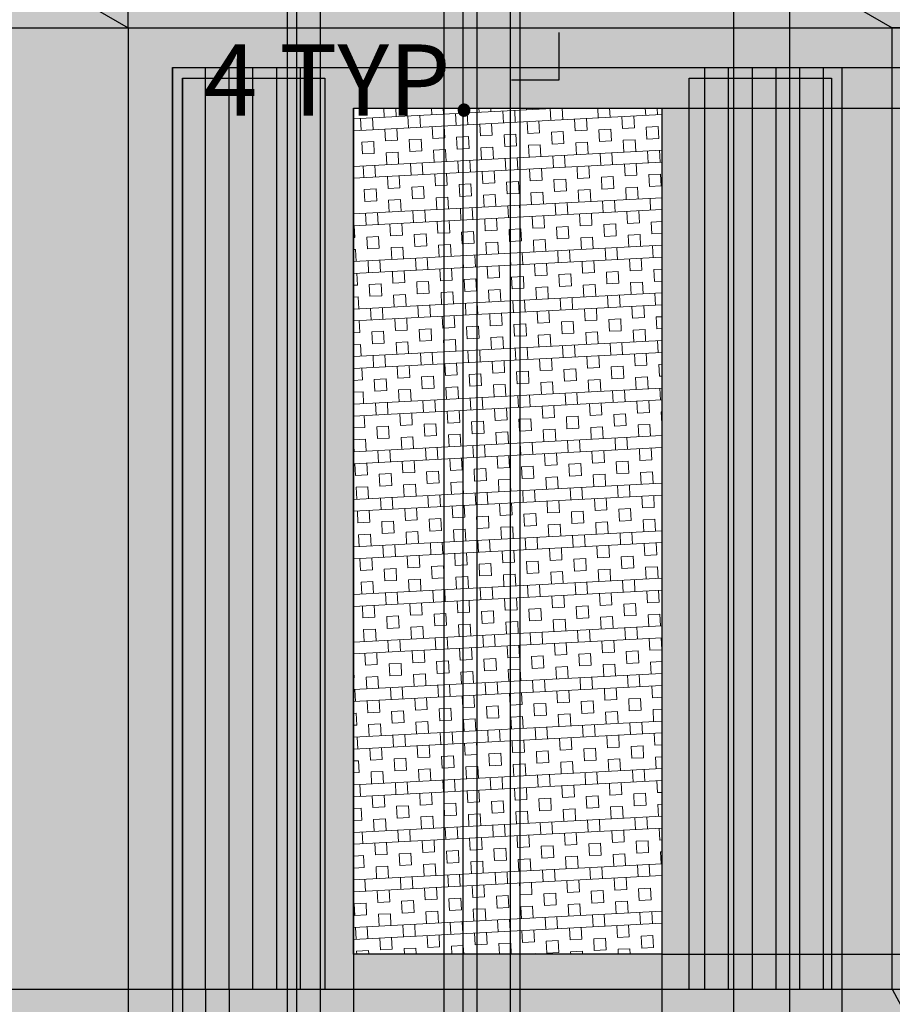
# Model space of a CAD drawing. Units: millimetres. Extents: x 131 to 845, y -20 to 1043.
# Tile 4 of 11: x 467 to 651, y 95 to 302. Entities that reach past the tile are written whole.
import ezdxf

# ---------------------------------------------------------------- set-up
doc = ezdxf.new("R2010")
doc.units = ezdxf.units.MM
doc.header["$MEASUREMENT"] = 0
for name, color, linetype, lineweight in [('A-ANNO-DIMS', 2, 'Continuous', 18), ('A-DOOR', 3, 'Continuous', 25), ('A-ELEV', 7, 'Continuous', 25), ('A-ELEV-PATT', 7, 'Continuous', 13), ('A-ELEV-SCRN', 4, 'Continuous', 13), ('A-GLAZ-PATT', 143, 'Continuous', 13)]:
    doc.layers.add(name, color=color, linetype=linetype, lineweight=lineweight)
doc.styles.get("Standard").update_dxf_attribs({"font": 'arial.ttf'})
doc.dimstyles.get("Standard").update_dxf_attribs({"dimtxt": 15, "dimasz": 10, "dimexe": 0.18, "dimexo": 0.0625, "dimgap": 5, "dimtad": 0, "dimtih": 1, "dimtoh": 1, "dimdec": 0, "dimzin": 0, "dimdsep": 46, "dimtxsty": 'Standard', "dimcen": 5, "dimadec": 0, "dimazin": 0, "dimtfac": 1, "dimtdec": 0, "dimtofl": 0, "dimtmove": 0, "dimatfit": 3, "dimfxl": 1, "dimtolj": 1, "dimtzin": 0, "dimarcsym": 0})

# ---------------------------------------------------------------- blocks, each defined once
blk = doc.blocks.new('*D9')
at = {"layer": 'A-ANNO-DIMS', "color": 0, "lineweight": -2, "transparency": 16777216}
for p, q in [((571.05, 313.91), (561.05, 313.91)), ((581.05, 313.22), (581.05, 314.09)), ((586.05, 313.22), (586.05, 314.09)), ((596.05, 313.91), (606.05, 313.91))]:
    blk.add_line(p, q, dxfattribs=at)
at = {"layer": 'A-ANNO-DIMS', "color": 0, "transparency": 16777216}
for points in [[(571.05, 315.58), (571.05, 312.24), (581.05, 313.91)], [(596.05, 315.58), (596.05, 312.24), (586.05, 313.91)]]:
    blk.add_solid(points, dxfattribs=at)
at = {"layer": 'Defpoints', "color": 0, "transparency": 16777216}
for p in [(581.05, 313.91), (581.05, 313.16), (586.05, 313.16)]:
    blk.add_point(p, dxfattribs=at)
at = {"layer": 'A-ANNO-DIMS', "color": 0, "transparency": 16777216, "insert": (409.24, 313.91), "char_height": 15, "attachment_point": 5}
blk.add_mtext('\\A1;BALCONY RAIL PANEL 5 TYP.', dxfattribs=at)
blk = doc.blocks.new('*D10')
at = {"layer": 'A-ANNO-DIMS', "color": 0, "lineweight": -2, "transparency": 16777216}
for p, q in [((580.3, 323.16), (580.3, 333.16)), ((580.98, 313.16), (580.12, 313.16)), ((580.98, 309.16), (580.12, 309.16)), ((580.3, 299.16), (580.3, 289.16)), ((580.3, 289.16), (570.3, 289.16))]:
    blk.add_line(p, q, dxfattribs=at)
at = {"layer": 'A-ANNO-DIMS', "color": 0, "transparency": 16777216}
for points in [[(578.63, 323.16), (581.96, 323.16), (580.3, 313.16)], [(578.63, 299.16), (581.96, 299.16), (580.3, 309.16)]]:
    blk.add_solid(points, dxfattribs=at)
at = {"layer": 'Defpoints', "color": 0, "transparency": 16777216}
for p in [(581.05, 313.16), (580.3, 309.16), (581.05, 309.16)]:
    blk.add_point(p, dxfattribs=at)
at = {"layer": 'A-ANNO-DIMS', "color": 0, "transparency": 16777216, "insert": (534.31, 289.16), "char_height": 15, "attachment_point": 5}
blk.add_mtext('\\A1;4 TYP.', dxfattribs=at)
blk = doc.blocks.new('*D50')
at = {"layer": 'A-ANNO-DIMS', "color": 0, "lineweight": -2, "transparency": 16777216}
for p, q in [((720.6, 488.6), (768.56, 488.6)), ((768.38, 478.6), (768.38, 287.12)), ((768.38, 70.31), (768.38, 261.79)), ((216.3, 60.31), (768.56, 60.31))]:
    blk.add_line(p, q, dxfattribs=at)
at = {"layer": 'A-ANNO-DIMS', "color": 0, "transparency": 16777216}
for points in [[(766.72, 478.6), (770.05, 478.6), (768.38, 488.6)], [(766.72, 70.31), (770.05, 70.31), (768.38, 60.31)]]:
    blk.add_solid(points, dxfattribs=at)
at = {"layer": 'Defpoints', "color": 0, "transparency": 16777216}
for p in [(720.53, 488.6), (768.38, 488.6), (216.23, 60.31)]:
    blk.add_point(p, dxfattribs=at)
at = {"layer": 'A-ANNO-DIMS', "color": 0, "transparency": 16777216, "insert": (768.38, 274.45), "char_height": 15, "attachment_point": 5}
blk.add_mtext('\\A1;428.3', dxfattribs=at)
blk = doc.blocks.new('*D51')
at = {"layer": 'A-ANNO-DIMS', "color": 0, "lineweight": -2, "transparency": 16777216}
for p, q in [((658.81, 488.53), (658.81, -10.22)), ((628.88, 312.6), (628.88, -10.22)), ((618.88, -10.04), (608.88, -10.04)), ((668.81, -10.04), (678.81, -10.04))]:
    blk.add_line(p, q, dxfattribs=at)
at = {"layer": 'A-ANNO-DIMS', "color": 0, "transparency": 16777216}
for points in [[(618.88, -8.37), (618.88, -11.7), (628.88, -10.04)], [(668.81, -8.37), (668.81, -11.7), (658.81, -10.04)]]:
    blk.add_solid(points, dxfattribs=at)
at = {"layer": 'Defpoints', "color": 0, "transparency": 16777216}
for p in [(658.81, 488.6), (628.88, 312.66), (658.81, -10.04)]:
    blk.add_point(p, dxfattribs=at)
at = {"layer": 'A-ANNO-DIMS', "color": 0, "transparency": 16777216, "insert": (715.07, -10.04), "char_height": 15, "attachment_point": 5}
blk.add_mtext('\\A1;29.923', dxfattribs=at)
blk = doc.blocks.new('*D52')
at = {"layer": 'A-ANNO-DIMS', "color": 0, "lineweight": -2, "transparency": 16777216}
for p, q in [((669.71, 488.53), (669.71, -10.22)), ((658.88, 312.6), (658.88, -10.22)), ((648.88, -10.04), (638.88, -10.04)), ((679.71, -10.04), (689.71, -10.04))]:
    blk.add_line(p, q, dxfattribs=at)
at = {"layer": 'A-ANNO-DIMS', "color": 0, "transparency": 16777216}
for points in [[(648.88, -8.37), (648.88, -11.7), (658.88, -10.04)], [(679.71, -8.37), (679.71, -11.7), (669.71, -10.04)]]:
    blk.add_solid(points, dxfattribs=at)
at = {"layer": 'Defpoints', "color": 0, "transparency": 16777216}
for p in [(669.71, 488.6), (658.88, 312.66), (669.71, -10.04)]:
    blk.add_point(p, dxfattribs=at)
at = {"layer": 'A-ANNO-DIMS', "color": 0, "transparency": 16777216, "insert": (725.2, -10.04), "char_height": 15, "attachment_point": 5}
blk.add_mtext('\\A1;10.825', dxfattribs=at)
blk = doc.blocks.new('*D60')
at = {"layer": 'A-ANNO-DIMS', "color": 0, "lineweight": -2, "transparency": 16777216}
for p, q in [((768.38, 333.16), (768.38, 343.16)), ((768.38, 343.16), (778.38, 343.16)), ((617.11, 323.16), (768.56, 323.16)), ((617.11, 305.16), (768.56, 305.16)), ((768.38, 295.16), (768.38, 285.16))]:
    blk.add_line(p, q, dxfattribs=at)
at = {"layer": 'A-ANNO-DIMS', "color": 0, "transparency": 16777216}
for points in [[(766.72, 333.16), (770.05, 333.16), (768.38, 323.16)], [(766.72, 295.16), (770.05, 295.16), (768.38, 305.16)]]:
    blk.add_solid(points, dxfattribs=at)
at = {"layer": 'Defpoints', "color": 0, "transparency": 16777216}
for p in [(617.05, 323.16), (768.38, 323.16), (617.05, 305.16)]:
    blk.add_point(p, dxfattribs=at)
at = {"layer": 'A-ANNO-DIMS', "color": 0, "transparency": 16777216, "insert": (793.44, 343.16), "char_height": 15, "attachment_point": 5}
blk.add_mtext('\\A1;18', dxfattribs=at)
blk = doc.blocks.new('*D61')
at = {"layer": 'A-ANNO-DIMS', "color": 0, "lineweight": -2, "transparency": 16777216}
for p, q in [((768.38, 333.16), (768.38, 343.16)), ((768.38, 343.16), (778.38, 343.16)), ((617.11, 323.16), (768.56, 323.16)), ((617.11, 319.16), (768.56, 319.16)), ((768.38, 309.16), (768.38, 299.16))]:
    blk.add_line(p, q, dxfattribs=at)
at = {"layer": 'A-ANNO-DIMS', "color": 0, "transparency": 16777216}
for points in [[(766.72, 333.16), (770.05, 333.16), (768.38, 323.16)], [(766.72, 309.16), (770.05, 309.16), (768.38, 319.16)]]:
    blk.add_solid(points, dxfattribs=at)
at = {"layer": 'Defpoints', "color": 0, "transparency": 16777216}
for p in [(617.05, 323.16), (768.38, 323.16), (617.05, 319.16)]:
    blk.add_point(p, dxfattribs=at)
at = {"layer": 'A-ANNO-DIMS', "color": 0, "transparency": 16777216, "insert": (788.57, 343.16), "char_height": 15, "attachment_point": 5}
blk.add_mtext('\\A1;4', dxfattribs=at)
blk = doc.blocks.new('*D62')
at = {"layer": 'A-ANNO-DIMS', "color": 0, "lineweight": -2, "transparency": 16777216}
for p, q in [((525.05, 459.74), (525.05, -10.22)), ((530.02, 454.68), (530.02, -10.22)), ((515.05, -10.04), (505.05, -10.04)), ((540.02, -10.04), (550.02, -10.04))]:
    blk.add_line(p, q, dxfattribs=at)
at = {"layer": 'A-ANNO-DIMS', "color": 0, "transparency": 16777216}
for points in [[(515.05, -8.37), (515.05, -11.7), (525.05, -10.04)], [(540.02, -8.37), (540.02, -11.7), (530.02, -10.04)]]:
    blk.add_solid(points, dxfattribs=at)
at = {"layer": 'Defpoints', "color": 0, "transparency": 16777216}
for p in [(525.05, 459.8), (530.02, 454.74), (530.02, -10.04)]:
    blk.add_point(p, dxfattribs=at)
at = {"layer": 'A-ANNO-DIMS', "color": 0, "transparency": 16777216, "insert": (580.63, -10.04), "char_height": 15, "attachment_point": 5}
blk.add_mtext('\\A1;4.977', dxfattribs=at)
blk = doc.blocks.new('*D65')
at = {"layer": 'A-ANNO-DIMS', "color": 0, "lineweight": -2, "transparency": 16777216}
for p, q in [((560.05, 439.74), (560.05, -10.22)), ((563.05, 439.74), (563.05, -10.22)), ((550.05, -10.04), (540.05, -10.04)), ((573.05, -10.04), (583.05, -10.04))]:
    blk.add_line(p, q, dxfattribs=at)
at = {"layer": 'A-ANNO-DIMS', "color": 0, "transparency": 16777216}
for points in [[(550.05, -8.37), (550.05, -11.7), (560.05, -10.04)], [(573.05, -8.37), (573.05, -11.7), (563.05, -10.04)]]:
    blk.add_solid(points, dxfattribs=at)
at = {"layer": 'Defpoints', "color": 0, "transparency": 16777216}
for p in [(560.05, 439.8), (563.05, 439.8), (563.05, -10.04)]:
    blk.add_point(p, dxfattribs=at)
at = {"layer": 'A-ANNO-DIMS', "color": 0, "transparency": 16777216, "insert": (592.96, -10.04), "char_height": 15, "attachment_point": 5}
blk.add_mtext('\\A1;3', dxfattribs=at)
blk = doc.blocks.new('*D67')
at = {"layer": 'A-ANNO-DIMS', "color": 0, "lineweight": -2, "transparency": 16777216}
for p, q in [((525.05, 459.74), (525.05, -10.22)), ((560.05, 439.74), (560.05, -10.22)), ((515.05, -10.04), (505.05, -10.04)), ((570.05, -10.04), (580.05, -10.04))]:
    blk.add_line(p, q, dxfattribs=at)
at = {"layer": 'A-ANNO-DIMS', "color": 0, "transparency": 16777216}
for points in [[(515.05, -8.37), (515.05, -11.7), (525.05, -10.04)], [(570.05, -8.37), (570.05, -11.7), (560.05, -10.04)]]:
    blk.add_solid(points, dxfattribs=at)
at = {"layer": 'Defpoints', "color": 0, "transparency": 16777216}
for p in [(525.05, 459.8), (560.05, 439.8), (560.05, -10.04)]:
    blk.add_point(p, dxfattribs=at)
at = {"layer": 'A-ANNO-DIMS', "color": 0, "transparency": 16777216, "insert": (542.55, -10.04), "char_height": 15, "attachment_point": 5}
blk.add_mtext('\\A1;35', dxfattribs=at)
blk = doc.blocks.new('*D68')
at = {"layer": 'A-ANNO-DIMS', "color": 0, "lineweight": -2, "transparency": 16777216}
for p, q in [((523.05, 305.1), (523.05, -10.22)), ((617.05, 305.1), (617.05, -10.22)), ((533.05, -10.04), (554.33, -10.04)), ((607.05, -10.04), (585.76, -10.04))]:
    blk.add_line(p, q, dxfattribs=at)
at = {"layer": 'A-ANNO-DIMS', "color": 0, "transparency": 16777216}
for points in [[(533.05, -8.37), (533.05, -11.7), (523.05, -10.04)], [(607.05, -8.37), (607.05, -11.7), (617.05, -10.04)]]:
    blk.add_solid(points, dxfattribs=at)
at = {"layer": 'Defpoints', "color": 0, "transparency": 16777216}
for p in [(523.05, 305.16), (617.05, 305.16), (617.05, -10.04)]:
    blk.add_point(p, dxfattribs=at)
at = {"layer": 'A-ANNO-DIMS', "color": 0, "transparency": 16777216, "insert": (570.05, -10.04), "char_height": 15, "attachment_point": 5}
blk.add_mtext('\\A1;94', dxfattribs=at)
blk = doc.blocks.new('*D69')
at = {"layer": 'A-ANNO-DIMS', "color": 0, "lineweight": -2, "transparency": 16777216}
for p, q in [((570.05, 303.56), (570.05, -10.22)), ((572.05, 303.56), (572.05, -10.22)), ((560.05, -10.04), (550.05, -10.04)), ((582.05, -10.04), (592.05, -10.04))]:
    blk.add_line(p, q, dxfattribs=at)
at = {"layer": 'A-ANNO-DIMS', "color": 0, "transparency": 16777216}
for points in [[(560.05, -8.37), (560.05, -11.7), (570.05, -10.04)], [(582.05, -8.37), (582.05, -11.7), (572.05, -10.04)]]:
    blk.add_solid(points, dxfattribs=at)
at = {"layer": 'Defpoints', "color": 0, "transparency": 16777216}
for p in [(570.05, 303.62), (572.05, 303.62), (572.05, -10.04)]:
    blk.add_point(p, dxfattribs=at)
at = {"layer": 'A-ANNO-DIMS', "color": 0, "transparency": 16777216, "insert": (616.63, -10.04), "char_height": 15, "attachment_point": 5}
blk.add_mtext('\\A1;2.00', dxfattribs=at)
blk = doc.blocks.new('*D70')
at = {"layer": 'A-ANNO-DIMS', "color": 0, "lineweight": -2, "transparency": 16777216}
for p, q in [((556.05, 309.1), (556.05, -10.22)), ((523.05, 305.1), (523.05, -10.22)), ((513.05, -10.04), (503.05, -10.04)), ((566.05, -10.04), (576.05, -10.04))]:
    blk.add_line(p, q, dxfattribs=at)
at = {"layer": 'A-ANNO-DIMS', "color": 0, "transparency": 16777216}
for points in [[(513.05, -8.37), (513.05, -11.7), (523.05, -10.04)], [(566.05, -8.37), (566.05, -11.7), (556.05, -10.04)]]:
    blk.add_solid(points, dxfattribs=at)
at = {"layer": 'Defpoints', "color": 0, "transparency": 16777216}
for p in [(556.05, 309.16), (523.05, 305.16), (556.05, -10.04)]:
    blk.add_point(p, dxfattribs=at)
at = {"layer": 'A-ANNO-DIMS', "color": 0, "transparency": 16777216, "insert": (539.55, -10.04), "char_height": 15, "attachment_point": 5}
blk.add_mtext('\\A1;33', dxfattribs=at)
blk = doc.blocks.new('*D71')
at = {"layer": 'A-ANNO-DIMS', "color": 0, "lineweight": -2, "transparency": 16777216}
for p, q in [((556.05, 309.1), (556.05, -10.22)), ((563.05, 309.1), (563.05, -10.22)), ((546.05, -10.04), (536.05, -10.04)), ((573.05, -10.04), (583.05, -10.04))]:
    blk.add_line(p, q, dxfattribs=at)
at = {"layer": 'A-ANNO-DIMS', "color": 0, "transparency": 16777216}
for points in [[(546.05, -8.37), (546.05, -11.7), (556.05, -10.04)], [(573.05, -8.37), (573.05, -11.7), (563.05, -10.04)]]:
    blk.add_solid(points, dxfattribs=at)
at = {"layer": 'Defpoints', "color": 0, "transparency": 16777216}
for p in [(556.05, 309.16), (563.05, 309.16), (563.05, -10.04)]:
    blk.add_point(p, dxfattribs=at)
at = {"layer": 'A-ANNO-DIMS', "color": 0, "transparency": 16777216, "insert": (592.9, -10.04), "char_height": 15, "attachment_point": 5}
blk.add_mtext('\\A1;7', dxfattribs=at)
blk = doc.blocks.new('*D72')
at = {"layer": 'A-ANNO-DIMS', "color": 0, "lineweight": -2, "transparency": 16777216}
for p, q in [((459.56, 300.1), (459.56, -10.22)), ((489.56, 300.1), (489.56, -10.22)), ((469.56, -10.04), (479.56, -10.04)), ((489.56, -10.04), (499.56, -10.04))]:
    blk.add_line(p, q, dxfattribs=at)
at = {"layer": 'A-ANNO-DIMS', "color": 0, "transparency": 16777216}
for points in [[(469.56, -8.37), (469.56, -11.7), (459.56, -10.04)], [(479.56, -8.37), (479.56, -11.7), (489.56, -10.04)]]:
    blk.add_solid(points, dxfattribs=at)
at = {"layer": 'Defpoints', "color": 0, "transparency": 16777216}
for p in [(459.56, 300.16), (489.56, 300.16), (489.56, -10.04)]:
    blk.add_point(p, dxfattribs=at)
at = {"layer": 'A-ANNO-DIMS', "color": 0, "transparency": 16777216, "insert": (515.27, -10.04), "char_height": 15, "attachment_point": 5}
blk.add_mtext('\\A1;30', dxfattribs=at)
blk = doc.blocks.new('*D75')
at = {"layer": 'A-ANNO-DIMS', "color": 0, "lineweight": -2, "transparency": 16777216}
for p, q in [((462.24, 1033.52), (452.24, 1033.52)), ((472.24, 310.22), (472.24, 1033.7)), ((489.56, 300.22), (489.56, 1033.7)), ((499.56, 1033.52), (509.56, 1033.52))]:
    blk.add_line(p, q, dxfattribs=at)
at = {"layer": 'A-ANNO-DIMS', "color": 0, "transparency": 16777216}
for points in [[(462.24, 1035.18), (462.24, 1031.85), (472.24, 1033.52)], [(499.56, 1035.18), (499.56, 1031.85), (489.56, 1033.52)]]:
    blk.add_solid(points, dxfattribs=at)
at = {"layer": 'Defpoints', "color": 0, "transparency": 16777216}
for p in [(489.56, 1033.52), (472.24, 310.16), (489.56, 300.16)]:
    blk.add_point(p, dxfattribs=at)
at = {"layer": 'A-ANNO-DIMS', "color": 0, "transparency": 16777216, "insert": (539.08, 1033.52), "char_height": 15, "attachment_point": 5}
blk.add_mtext('\\A1;17.32', dxfattribs=at)
blk = doc.blocks.new('*D76')
at = {"layer": 'A-ANNO-DIMS', "color": 0, "lineweight": -2, "transparency": 16777216}
for p, q in [((768.38, 320.16), (768.38, 330.16)), ((472.3, 310.16), (768.56, 310.16)), ((489.62, 300.16), (768.56, 300.16)), ((768.38, 290.16), (768.38, 280.16)), ((768.38, 280.16), (758.38, 280.16))]:
    blk.add_line(p, q, dxfattribs=at)
at = {"layer": 'A-ANNO-DIMS', "color": 0, "transparency": 16777216}
for points in [[(766.72, 320.16), (770.05, 320.16), (768.38, 310.16)], [(766.72, 290.16), (770.05, 290.16), (768.38, 300.16)]]:
    blk.add_solid(points, dxfattribs=at)
at = {"layer": 'Defpoints', "color": 0, "transparency": 16777216}
for p in [(472.24, 310.16), (489.56, 300.16), (768.38, 300.16)]:
    blk.add_point(p, dxfattribs=at)
at = {"layer": 'A-ANNO-DIMS', "color": 0, "transparency": 16777216, "insert": (743.37, 280.16), "char_height": 15, "attachment_point": 5}
blk.add_mtext('\\A1;10', dxfattribs=at)
blk = doc.blocks.new('*D77')
at = {"layer": 'A-ANNO-DIMS', "color": 0, "lineweight": -2, "transparency": 16777216}
for p, q in [((648.88, 1033.52), (638.88, 1033.52)), ((658.88, 312.72), (658.88, 1033.7)), ((680.53, 300.22), (680.53, 1033.7)), ((690.53, 1033.52), (700.53, 1033.52))]:
    blk.add_line(p, q, dxfattribs=at)
at = {"layer": 'A-ANNO-DIMS', "color": 0, "transparency": 16777216}
for points in [[(648.88, 1035.18), (648.88, 1031.85), (658.88, 1033.52)], [(690.53, 1035.18), (690.53, 1031.85), (680.53, 1033.52)]]:
    blk.add_solid(points, dxfattribs=at)
at = {"layer": 'Defpoints', "color": 0, "transparency": 16777216}
for p in [(680.53, 1033.52), (658.88, 312.66), (680.53, 300.16)]:
    blk.add_point(p, dxfattribs=at)
at = {"layer": 'A-ANNO-DIMS', "color": 0, "transparency": 16777216, "insert": (731.03, 1033.52), "char_height": 15, "attachment_point": 5}
blk.add_mtext('\\A1;21.65', dxfattribs=at)
blk = doc.blocks.new('*D79')
at = {"layer": 'A-ANNO-DIMS', "color": 0, "lineweight": -2, "transparency": 16777216}
for p, q in [((489.56, 300.1), (489.56, -10.22)), ((498.91, 291.72), (498.91, -10.22)), ((479.56, -10.04), (469.56, -10.04)), ((508.91, -10.04), (518.91, -10.04))]:
    blk.add_line(p, q, dxfattribs=at)
at = {"layer": 'A-ANNO-DIMS', "color": 0, "transparency": 16777216}
for points in [[(479.56, -8.37), (479.56, -11.7), (489.56, -10.04)], [(508.91, -8.37), (508.91, -11.7), (498.91, -10.04)]]:
    blk.add_solid(points, dxfattribs=at)
at = {"layer": 'Defpoints', "color": 0, "transparency": 16777216}
for p in [(489.56, 300.16), (498.91, 291.78), (498.91, -10.04)]:
    blk.add_point(p, dxfattribs=at)
at = {"layer": 'A-ANNO-DIMS', "color": 0, "transparency": 16777216, "insert": (549.23, -10.04), "char_height": 15, "attachment_point": 5}
blk.add_mtext('\\A1;9.349', dxfattribs=at)
blk = doc.blocks.new('*D80')
at = {"layer": 'A-ANNO-DIMS', "color": 0, "lineweight": -2, "transparency": 16777216}
for p, q in [((498.91, 291.72), (498.91, -10.22)), ((639.87, 291.72), (639.87, -10.22)), ((508.91, -10.04), (533.96, -10.04)), ((629.87, -10.04), (604.81, -10.04))]:
    blk.add_line(p, q, dxfattribs=at)
at = {"layer": 'A-ANNO-DIMS', "color": 0, "transparency": 16777216}
for points in [[(508.91, -8.37), (508.91, -11.7), (498.91, -10.04)], [(629.87, -8.37), (629.87, -11.7), (639.87, -10.04)]]:
    blk.add_solid(points, dxfattribs=at)
at = {"layer": 'Defpoints', "color": 0, "transparency": 16777216}
for p in [(498.91, 291.78), (639.87, 291.78), (639.87, -10.04)]:
    blk.add_point(p, dxfattribs=at)
at = {"layer": 'A-ANNO-DIMS', "color": 0, "transparency": 16777216, "insert": (569.39, -10.04), "char_height": 15, "attachment_point": 5}
blk.add_mtext('\\A1;140.96', dxfattribs=at)
blk = doc.blocks.new('*D81')
at = {"layer": 'A-ANNO-DIMS', "color": 0, "lineweight": -2, "transparency": 16777216}
for p, q in [((498.97, 291.78), (768.56, 291.78)), ((768.38, 281.78), (768.38, 207.46)), ((768.38, 107.81), (768.38, 182.13)), ((498.97, 97.81), (768.56, 97.81))]:
    blk.add_line(p, q, dxfattribs=at)
at = {"layer": 'A-ANNO-DIMS', "color": 0, "transparency": 16777216}
for points in [[(766.72, 281.78), (770.05, 281.78), (768.38, 291.78)], [(766.72, 107.81), (770.05, 107.81), (768.38, 97.81)]]:
    blk.add_solid(points, dxfattribs=at)
at = {"layer": 'Defpoints', "color": 0, "transparency": 16777216}
for p in [(498.91, 291.78), (768.38, 291.78), (498.91, 97.81)]:
    blk.add_point(p, dxfattribs=at)
at = {"layer": 'A-ANNO-DIMS', "color": 0, "transparency": 16777216, "insert": (768.38, 194.8), "char_height": 15, "attachment_point": 5}
blk.add_mtext('\\A1;193.97', dxfattribs=at)
blk = doc.blocks.new('*D82')
at = {"layer": 'A-ANNO-DIMS', "color": 0, "lineweight": -2, "transparency": 16777216}
for p, q in [((537.05, 283.2), (537.05, -10.22)), ((601.99, 283.2), (601.99, -10.22)), ((527.05, -10.04), (517.05, -10.04)), ((611.99, -10.04), (621.99, -10.04))]:
    blk.add_line(p, q, dxfattribs=at)
at = {"layer": 'A-ANNO-DIMS', "color": 0, "transparency": 16777216}
for points in [[(527.05, -8.37), (527.05, -11.7), (537.05, -10.04)], [(611.99, -8.37), (611.99, -11.7), (601.99, -10.04)]]:
    blk.add_solid(points, dxfattribs=at)
at = {"layer": 'Defpoints', "color": 0, "transparency": 16777216}
for p in [(537.05, 283.26), (601.99, 283.26), (601.99, -10.04)]:
    blk.add_point(p, dxfattribs=at)
at = {"layer": 'A-ANNO-DIMS', "color": 0, "transparency": 16777216, "insert": (569.52, -10.04), "char_height": 15, "attachment_point": 5}
blk.add_mtext('\\A1;64.95', dxfattribs=at)
blk = doc.blocks.new('*D83')
at = {"layer": 'A-ANNO-DIMS', "color": 0, "lineweight": -2, "transparency": 16777216}
for p, q in [((602.06, 283.26), (768.56, 283.26)), ((768.38, 273.26), (768.38, 206.85)), ((768.38, 115.12), (768.38, 181.53)), ((602.06, 105.12), (768.56, 105.12))]:
    blk.add_line(p, q, dxfattribs=at)
at = {"layer": 'A-ANNO-DIMS', "color": 0, "transparency": 16777216}
for points in [[(766.72, 273.26), (770.05, 273.26), (768.38, 283.26)], [(766.72, 115.12), (770.05, 115.12), (768.38, 105.12)]]:
    blk.add_solid(points, dxfattribs=at)
at = {"layer": 'Defpoints', "color": 0, "transparency": 16777216}
for p in [(601.99, 283.26), (768.38, 283.26), (601.99, 105.12)]:
    blk.add_point(p, dxfattribs=at)
at = {"layer": 'A-ANNO-DIMS', "color": 0, "transparency": 16777216, "insert": (768.38, 194.19), "char_height": 15, "attachment_point": 5}
blk.add_mtext('\\A1;178.14', dxfattribs=at)
blk = doc.blocks.new('*D84')
at = {"layer": 'A-ANNO-DIMS', "color": 0, "lineweight": -2, "transparency": 16777216}
for p, q in [((500.99, 289.46), (500.99, -10.22)), ((537.05, 283.2), (537.05, -10.22)), ((510.99, -10.04), (527.05, -10.04)), ((537.05, -10.04), (547.05, -10.04))]:
    blk.add_line(p, q, dxfattribs=at)
at = {"layer": 'A-ANNO-DIMS', "color": 0, "transparency": 16777216}
for points in [[(510.99, -8.37), (510.99, -11.7), (500.99, -10.04)], [(527.05, -8.37), (527.05, -11.7), (537.05, -10.04)]]:
    blk.add_solid(points, dxfattribs=at)
at = {"layer": 'Defpoints', "color": 0, "transparency": 16777216}
for p in [(500.99, 289.52), (537.05, 283.26), (537.05, -10.04)]:
    blk.add_point(p, dxfattribs=at)
at = {"layer": 'A-ANNO-DIMS', "color": 0, "transparency": 16777216, "insert": (577.41, -10.04), "char_height": 15, "attachment_point": 5}
blk.add_mtext('\\A1;36.05', dxfattribs=at)
blk = doc.blocks.new('*D85')
at = {"layer": 'A-ANNO-DIMS', "color": 0, "lineweight": -2, "transparency": 16777216}
for p, q in [((768.38, 301.78), (768.38, 311.78)), ((768.38, 311.78), (778.38, 311.78)), ((639.93, 291.78), (768.56, 291.78)), ((602.06, 283.26), (768.56, 283.26)), ((768.38, 273.26), (768.38, 263.26))]:
    blk.add_line(p, q, dxfattribs=at)
at = {"layer": 'A-ANNO-DIMS', "color": 0, "transparency": 16777216}
for points in [[(766.72, 301.78), (770.05, 301.78), (768.38, 291.78)], [(766.72, 273.26), (770.05, 273.26), (768.38, 283.26)]]:
    blk.add_solid(points, dxfattribs=at)
at = {"layer": 'Defpoints', "color": 0, "transparency": 16777216}
for p in [(639.87, 291.78), (768.38, 291.78), (601.99, 283.26)]:
    blk.add_point(p, dxfattribs=at)
at = {"layer": 'A-ANNO-DIMS', "color": 0, "transparency": 16777216, "insert": (808.63, 311.78), "char_height": 15, "attachment_point": 5}
blk.add_mtext('\\A1;8.522', dxfattribs=at)
blk = doc.blocks.new('*D86')
at = {"layer": 'A-ANNO-DIMS', "color": 0, "lineweight": -2, "transparency": 16777216}
for p, q in [((505.87, 97.75), (505.87, -10.22)), ((510.87, 97.75), (510.87, -10.22)), ((495.87, -10.04), (485.87, -10.04)), ((520.87, -10.04), (530.87, -10.04))]:
    blk.add_line(p, q, dxfattribs=at)
at = {"layer": 'A-ANNO-DIMS', "color": 0, "transparency": 16777216}
for points in [[(495.87, -8.37), (495.87, -11.7), (505.87, -10.04)], [(520.87, -8.37), (520.87, -11.7), (510.87, -10.04)]]:
    blk.add_solid(points, dxfattribs=at)
at = {"layer": 'Defpoints', "color": 0, "transparency": 16777216}
for p in [(505.87, 97.81), (510.87, 97.81), (510.87, -10.04)]:
    blk.add_point(p, dxfattribs=at)
at = {"layer": 'A-ANNO-DIMS', "color": 0, "transparency": 16777216, "insert": (540.84, -10.04), "char_height": 15, "attachment_point": 5}
blk.add_mtext('\\A1;5', dxfattribs=at)
blk = doc.blocks.new('*D99')
at = {"layer": 'A-ANNO-DIMS', "color": 0, "lineweight": -2, "transparency": 16777216}
for p, q in [((449.56, 833.53), (449.56, -10.22)), ((446.56, 818.53), (446.56, -10.22)), ((436.56, -10.04), (426.56, -10.04)), ((459.56, -10.04), (469.56, -10.04))]:
    blk.add_line(p, q, dxfattribs=at)
at = {"layer": 'A-ANNO-DIMS', "color": 0, "transparency": 16777216}
for points in [[(436.56, -8.37), (436.56, -11.7), (446.56, -10.04)], [(459.56, -8.37), (459.56, -11.7), (449.56, -10.04)]]:
    blk.add_solid(points, dxfattribs=at)
at = {"layer": 'Defpoints', "color": 0, "transparency": 16777216}
for p in [(449.56, 833.6), (446.56, 818.6), (449.56, -10.04)]:
    blk.add_point(p, dxfattribs=at)
at = {"layer": 'A-ANNO-DIMS', "color": 0, "transparency": 16777216, "insert": (479.47, -10.04), "char_height": 15, "attachment_point": 5}
blk.add_mtext('\\A1;3', dxfattribs=at)

msp = doc.modelspace()

# ---------------------------------------------------------------- hatches: boundary and pattern name
at = {"layer": 'A-ELEV-PATT', "transparency": 33554681}
h = msp.add_hatch(color=256, dxfattribs=at)
h.set_gradient(color1=(255, 255, 255), color2=(199, 200, 202), name='INVSPHERICAL')
h.paths.add_polyline_path([(459.5586, 310.1596), (472.2381, 310.1596), (489.5586, 300.1596), (650.5349, 300.1596), (628.8842, 312.6596), (628.8842, 488.5953), (459.5586, 488.5953)])
h.paths.add_polyline_path([(525.0467, 459.8046), (615.0467, 459.8046), (615.0467, 323.1596), (617.0467, 323.1596), (617.0467, 319.1596), (615.0467, 319.1596), (615.0467, 309.1596), (617.0467, 309.1596), (617.0467, 305.1596), (572.0467, 305.1596), (572.0453, 303.6234), (570.0467, 303.6234), (570.0467, 305.1596), (525.0467, 305.1596), (523.0467, 305.1596), (523.0467, 309.1596), (525.0467, 309.1596), (525.0467, 319.1596), (523.0467, 319.1596), (523.0467, 323.1596), (525.0467, 323.1596)], flags=16)
h.paths.add_polyline_path([(530.0467, 454.8046), (550.0467, 454.8046), (550.0467, 423.2044), (530.0467, 423.2044)], flags=0)
h.paths.add_polyline_path([(530.0467, 418.2044), (550.0467, 418.2044), (550.0467, 386.7044), (530.0467, 386.7044)], flags=0)
h.paths.add_polyline_path([(560.0467, 439.8046), (563.0467, 439.8046), (563.0467, 328.8046), (560.0467, 328.8046)], flags=0)
h.paths.add_polyline_path([(530.0467, 381.7044), (550.0467, 381.7044), (550.0467, 350.2044), (530.0467, 350.2044)], flags=0)
h.paths.add_polyline_path([(554.0467, 319.1596), (554.0467, 315.1596), (540.0467, 315.1596), (540.0467, 313.7044), (530.0467, 313.7044), (530.0467, 319.1596)], flags=0)
h.paths.add_polyline_path([(556.0467, 319.1596), (561.0467, 319.1596), (561.0467, 315.1596), (556.0467, 315.1596)], flags=0)
h.paths.add_polyline_path([(563.0467, 319.1596), (568.0467, 319.1596), (568.0467, 315.1596), (563.0467, 315.1596)], flags=0)
h.paths.add_polyline_path([(556.0467, 313.1596), (561.0467, 313.1596), (561.0467, 309.1596), (556.0467, 309.1596)], flags=0)
h.paths.add_polyline_path([(563.0467, 313.1596), (568.0467, 313.1596), (568.0467, 309.1596), (563.0467, 309.1596)], flags=0)
h.paths.add_polyline_path([(574.0467, 319.1596), (579.0467, 319.1596), (579.0467, 315.1596), (574.1854, 315.1596), (574.1854, 313.1596), (579.0467, 313.1596), (579.0467, 309.1596), (574.0467, 309.1596), (574.0467, 313.1596), (574.1854, 315.1596), (574.0467, 315.1596)], flags=0)
h.paths.add_polyline_path([(581.0467, 319.1596), (586.0467, 319.1596), (586.0467, 315.1596), (581.0467, 315.1596)], flags=0)
h.paths.add_polyline_path([(581.0467, 313.1596), (586.0467, 313.1596), (586.0467, 309.1596), (581.0467, 309.1596)], flags=0)
h = msp.add_hatch(color=256, dxfattribs=at)
h.set_gradient(color1=(79, 2, 22), color2=(153, 133, 76), name='SPHERICAL')
h.paths.add_polyline_path([(459.5586, 310.1596), (459.5586, 300.1596), (489.5586, 300.1596), (472.2381, 310.1596)])
h.paths.add_polyline_path([(658.8842, 312.6596), (628.8842, 312.6596), (650.5349, 300.1596), (680.5349, 300.1596)])
h = msp.add_hatch(color=256, dxfattribs=at)
h.set_gradient(color1=(255, 255, 255), color2=(199, 200, 202), name='INVSPHERICAL')
h.paths.add_polyline_path([(489.5586, 300.1596), (459.5586, 300.1596), (459.5586, 252.07), (459.5586, 97.8131), (489.5586, 97.8131)])
h.paths.add_polyline_path([(680.5349, 300.1596), (650.5349, 300.1596), (650.5349, 97.8131), (680.5349, 97.8131)])
h.paths.add_polyline_path([(658.5215, 82.8131), (459.5586, 82.8131), (459.5586, 67.8131), (658.5215, 67.8131)])
h.paths.add_polyline_path([(663.9762, 52.8131), (459.5586, 52.8131), (459.5586, 37.8131), (663.9762, 37.8131)])
h.paths.add_polyline_path([(680.5349, 97.8131), (650.5349, 97.8131), (658.5215, 82.8131), (658.5215, 67.8131), (661.2489, 60.3131), (680.5349, 60.3131)])
h = msp.add_hatch(color=256, dxfattribs=at)
h.set_gradient(color1=(153, 95, 76), color2=(79, 2, 22), name='SPHERICAL')
h.paths.add_polyline_path([(530.9938, 97.8131), (607.7215, 97.8131), (607.7215, 289.5229), (610.9926, 289.5229), (610.9926, 291.7824), (525.8699, 291.7824), (525.8699, 289.5229), (530.9938, 289.5229)], flags=17)
h.paths.add_polyline_path([(537.0455, 283.2603), (601.9946, 283.2603), (601.9946, 105.1179), (537.0455, 105.1179)], flags=16)
h.paths.add_polyline_path([(489.5586, 97.8131), (498.9074, 97.8131), (498.9074, 291.7824), (639.8713, 291.7824), (639.8713, 97.8131), (650.5349, 97.8131), (650.5349, 300.1596), (489.5586, 300.1596)])
h = msp.add_hatch(color=256, dxfattribs=at)
h.set_gradient(color1=(153, 133, 76), color2=(241, 235, 31), name='SPHERICAL')
h.paths.add_polyline_path([(505.8699, 289.5229), (500.9938, 289.5229), (500.9938, 97.8131), (505.8699, 97.8131)], flags=17)
h.paths.add_polyline_path([(510.8699, 289.5229), (505.8699, 289.5229), (505.8699, 97.8131), (510.8699, 97.8131)])
h.paths.add_polyline_path([(515.8699, 289.5229), (510.8699, 289.5229), (510.8699, 97.8131), (515.8699, 97.8131)])
h.paths.add_polyline_path([(520.8699, 289.5229), (515.8699, 289.5229), (515.8699, 97.8131), (520.8699, 97.8131)])
h.paths.add_polyline_path([(525.8699, 289.5229), (520.8699, 289.5229), (520.8699, 97.8131), (525.8699, 97.8131)])
h.paths.add_polyline_path([(530.9938, 289.5229), (525.8699, 289.5229), (525.8699, 97.8131), (530.9938, 97.8131)])
h.paths.add_polyline_path([(610.9926, 289.5229), (607.7215, 289.5229), (607.7215, 97.8131), (610.9926, 97.8131)])
h.paths.add_polyline_path([(615.9926, 289.5229), (610.9926, 289.5229), (610.9926, 97.8131), (615.9926, 97.8131)])
h.paths.add_polyline_path([(620.9926, 289.5229), (615.9926, 289.5229), (615.9926, 97.8131), (620.9926, 97.8131)])
h.paths.add_polyline_path([(625.9926, 289.5229), (620.9926, 289.5229), (620.9926, 97.8131), (625.9926, 97.8131)])
h.paths.add_polyline_path([(630.9926, 289.5229), (625.9926, 289.5229), (625.9926, 97.8131), (630.9926, 97.8131)])
h.paths.add_polyline_path([(635.9926, 289.5229), (630.9926, 289.5229), (630.9926, 97.8131), (635.9926, 97.8131)])
h.paths.add_polyline_path([(639.8713, 291.7824), (635.9926, 291.7824), (635.9926, 289.5229), (637.7215, 289.5229), (637.7215, 97.8131), (639.8713, 97.8131)])
h.paths.add_polyline_path([(637.7215, 289.5229), (635.9926, 289.5229), (635.9926, 97.8131), (637.7215, 97.8131)], flags=17)
h.paths.add_polyline_path([(500.9938, 289.5229), (505.8699, 289.5229), (505.8699, 291.7824), (498.9074, 291.7824), (498.9074, 97.8131), (500.9938, 97.8131)])
h.paths.add_polyline_path([(510.8699, 291.7824), (505.8699, 291.7824), (505.8699, 289.5229), (510.8699, 289.5229)])
h.paths.add_polyline_path([(515.8699, 291.7824), (510.8699, 291.7824), (510.8699, 289.5229), (515.8699, 289.5229)])
h.paths.add_polyline_path([(520.8699, 291.7824), (515.8699, 291.7824), (515.8699, 289.5229), (520.8699, 289.5229)])
h.paths.add_polyline_path([(525.8699, 291.7824), (520.8699, 291.7824), (520.8699, 289.5229), (525.8699, 289.5229)])
h.paths.add_polyline_path([(615.9926, 291.7824), (610.9926, 291.7824), (610.9926, 289.5229), (615.9926, 289.5229)])
h.paths.add_polyline_path([(620.9926, 291.7824), (615.9926, 291.7824), (615.9926, 289.5229), (620.9926, 289.5229)])
h.paths.add_polyline_path([(625.9926, 291.7824), (620.9926, 291.7824), (620.9926, 289.5229), (625.9926, 289.5229)])
h.paths.add_polyline_path([(630.9926, 291.7824), (625.9926, 291.7824), (625.9926, 289.5229), (630.9926, 289.5229)])
h.paths.add_polyline_path([(635.9926, 291.7824), (630.9926, 291.7824), (630.9926, 289.5229), (635.9926, 289.5229)])
at = {"layer": 'A-ELEV-SCRN'}
h = msp.add_hatch(dxfattribs=at)
h.set_pattern_fill('BOX', color=256, scale=10, angle=93)
h.paths.add_polyline_path([(601.9946, 283.2603), (537.0455, 283.2603), (537.0455, 105.1179), (601.9946, 105.1179)])
at = {"layer": 'A-GLAZ-PATT'}
h = msp.add_hatch(color=256, dxfattribs=at)
h.dxf.hatch_style = 1
h.paths.add_polyline_path([(658.8074, 488.5953), (628.8842, 488.5953), (628.8842, 312.6596), (658.8842, 312.6596)])
h.paths.add_polyline_path([(650.5349, 97.8131), (459.5586, 97.8131), (459.5586, 82.8131), (658.5215, 82.8131)])
h.paths.add_polyline_path([(658.5215, 67.8131), (459.5586, 67.8131), (459.5586, 52.8131), (663.9762, 52.8131)])

# ---------------------------------------------------------------- linework, layer by layer
at = {"layer": 'A-DOOR'}
for p, q in [((505.8699, 97.8131), (505.8699, 291.7824)), ((510.8699, 97.8131), (510.8699, 291.7824)), ((515.8699, 97.8131), (515.8699, 291.7824)), ((520.8699, 97.8131), (520.8699, 291.7824)), ((525.8699, 97.8131), (525.8699, 291.7824)), ((610.9926, 291.7824), (610.9926, 97.8131)), ((615.9926, 291.7824), (615.9926, 97.8131)), ((620.9926, 291.7824), (620.9926, 97.8131)), ((625.9926, 291.7824), (625.9926, 97.8131)), ((630.9926, 291.7824), (630.9926, 97.8131)), ((635.9926, 291.7824), (635.9926, 97.8131))]:
    msp.add_line(p, q, dxfattribs=at)
for points in [[(498.9074, 97.8131), (498.9074, 291.7824), (639.8713, 291.7824), (639.8713, 97.8131)], [(500.9938, 97.8131), (500.9938, 289.5229), (530.9938, 289.5229), (530.9938, 97.8131)], [(607.7215, 97.8131), (607.7215, 289.5229), (637.7215, 289.5229), (637.7215, 97.8131)]]:
    msp.add_lwpolyline(points, dxfattribs=at)
msp.add_lwpolyline([(537.0455, 283.2603), (601.9946, 283.2603), (601.9946, 105.1179), (537.0455, 105.1179)], close=True, dxfattribs=at)
at = {"layer": 'A-ELEV'}
for p, q in [((628.8842, 312.6596), (650.5349, 300.1596)), ((472.2381, 310.1596), (489.5586, 300.1596)), ((459.5586, 300.1596), (489.5586, 300.1596)), ((489.5586, 300.1596), (489.5586, 97.8131)), ((489.5586, 300.1596), (650.5349, 300.1596)), ((680.5349, 300.1596), (650.5349, 300.1596)), ((650.5349, 97.8131), (650.5349, 300.1596)), ((459.5586, 97.8131), (650.5349, 97.8131)), ((650.5349, 97.8131), (658.5215, 82.8131))]:
    msp.add_line(p, q, dxfattribs=at)

# ---------------------------------------------------------------- dimensions: what is measured, and where the dimension line sits
at = {"layer": 'A-ANNO-DIMS'}
for base, p1, p2, override, picture, middle in [((489.5586, 1033.5163), (472.2381, 310.1596), (489.5586, 300.1596), {"dimdec": 2, "dimlfac": 1, "dimrnd": 0, "dimzin": 0, "dimdsep": 46, "dimlunit": 2}, '*D75', (539.0845, 1033.5163)), ((680.5349, 1033.5163), (658.8842, 312.6596), (680.5349, 300.1596), {"dimdec": 2, "dimlfac": 1, "dimrnd": 0, "dimzin": 0, "dimdsep": 46, "dimlunit": 2}, '*D77', (731.0277, 1033.5163)), ((449.5586, -10.0369), (446.5586, 818.5953), (449.5586, 833.5953), {"dimdec": 0, "dimlfac": 1, "dimrnd": 0, "dimzin": 0, "dimdsep": 46, "dimlunit": 2}, '*D99', (479.4699, -10.0369)), ((658.8074, -10.0369), (628.8842, 312.6596), (658.8074, 488.5953), {"dimdec": 3, "dimlfac": 1, "dimrnd": 0, "dimzin": 0, "dimdsep": 46, "dimlunit": 2}, '*D51', (715.0711, -10.0369)), ((669.7096, -10.0369), (658.8842, 312.6596), (669.7096, 488.5953), {"dimdec": 3, "dimlfac": 1, "dimrnd": 0, "dimzin": 0, "dimdsep": 46, "dimlunit": 2}, '*D52', (725.1956, -10.0369)), ((530.0241, -10.0369), (525.0467, 459.8046), (530.0241, 454.7401), {"dimdec": 3, "dimlfac": 1, "dimrnd": 0, "dimzin": 0, "dimdsep": 46, "dimlunit": 2}, '*D62', (580.6346, -10.0369)), ((560.0467, -10.0369), (525.0467, 459.8046), (560.0467, 439.8046), {"dimdec": 0, "dimlfac": 1, "dimrnd": 0, "dimzin": 0, "dimdsep": 46, "dimlunit": 2}, '*D67', (542.5467, -10.0369)), ((563.0467, -10.0369), (560.0467, 439.8046), (563.0467, 439.8046), {"dimdec": 0, "dimlfac": 1, "dimrnd": 0, "dimzin": 0, "dimdsep": 46, "dimlunit": 2}, '*D65', (592.9581, -10.0369)), ((556.0467, -10.0369), (523.0467, 305.1596), (556.0467, 309.1596), {"dimdec": 0, "dimlfac": 1, "dimrnd": 0, "dimzin": 0, "dimdsep": 46, "dimlunit": 2}, '*D70', (539.5467, -10.0369)), ((563.0467, -10.0369), (556.0467, 309.1596), (563.0467, 309.1596), {"dimdec": 0, "dimlfac": 1, "dimrnd": 0, "dimzin": 0, "dimdsep": 46, "dimlunit": 2}, '*D71', (592.9018, -10.0369)), ((617.0467, -10.0369), (523.0467, 305.1596), (617.0467, 305.1596), {"dimdec": 0, "dimlfac": 1, "dimrnd": 0, "dimzin": 0, "dimdsep": 46, "dimlunit": 2}, '*D68', (570.0467, -10.0369)), ((572.0453, -10.0369), (570.0467, 303.6234), (572.0453, 303.6234), {"dimdec": 2, "dimlfac": 1, "dimrnd": 0, "dimzin": 0, "dimdsep": 46, "dimlunit": 2}, '*D69', (616.6292, -10.0369)), ((489.5586, -10.0369), (459.5586, 300.1596), (489.5586, 300.1596), {"dimdec": 0, "dimlfac": 1, "dimrnd": 0, "dimzin": 0, "dimdsep": 46, "dimlunit": 2}, '*D72', (515.2714, -10.0369)), ((498.9074, -10.0369), (489.5586, 300.1596), (498.9074, 291.7824), {"dimdec": 3, "dimlfac": 1, "dimrnd": 0, "dimzin": 0, "dimdsep": 46, "dimlunit": 2}, '*D79', (549.2314, -10.0369)), ((639.8713, -10.0369), (498.9074, 291.7824), (639.8713, 291.7824), {"dimdec": 2, "dimlfac": 1, "dimrnd": 0, "dimzin": 0, "dimdsep": 46, "dimlunit": 2}, '*D80', (569.3893, -10.0369)), ((537.0455, -10.0369), (500.9938, 289.5229), (537.0455, 283.2603), {"dimdec": 2, "dimlfac": 1, "dimrnd": 0, "dimzin": 0, "dimdsep": 46, "dimlunit": 2}, '*D84', (577.4053, -10.0369)), ((601.9946, -10.0369), (537.0455, 283.2603), (601.9946, 283.2603), {"dimdec": 2, "dimlfac": 1, "dimrnd": 0, "dimzin": 0, "dimdsep": 46, "dimlunit": 2}, '*D82', (569.5201, -10.0369)), ((510.8699, -10.0369), (505.8699, 97.8131), (510.8699, 97.8131), {"dimdec": 0, "dimlfac": 1, "dimrnd": 0, "dimzin": 0, "dimdsep": 46, "dimlunit": 2}, '*D86', (540.8426, -10.0369))]:
    dim = msp.add_linear_dim(base=base, p1=p1, p2=p2, dimstyle='Standard', override=override, dxfattribs=at)
    dim.commit()
    dim.dimension.update_dxf_attribs({"geometry": picture, "text_midpoint": middle})
for base, p1, p2, override, picture, middle in [((768.3849, 488.5953), (216.2327, 60.3131), (720.5349, 488.5953), {"dimdec": 1, "dimlfac": 1, "dimrnd": 0, "dimzin": 0, "dimdsep": 46, "dimlunit": 2}, '*D50', (768.3849, 274.4542)), ((768.3849, 323.1596), (617.0467, 305.1596), (617.0467, 323.1596), {"dimdec": 0, "dimlfac": 1, "dimrnd": 0, "dimzin": 0, "dimdsep": 46, "dimlunit": 2}, '*D60', (793.4377, 343.1596)), ((768.3849, 323.1596), (617.0467, 319.1596), (617.0467, 323.1596), {"dimdec": 0, "dimlfac": 1, "dimrnd": 0, "dimzin": 0, "dimdsep": 46, "dimlunit": 2}, '*D61', (788.5725, 343.1596)), ((768.3849, 300.1596), (472.2381, 310.1596), (489.5586, 300.1596), {"dimdec": 0, "dimlfac": 1, "dimrnd": 0, "dimzin": 0, "dimdsep": 46, "dimlunit": 2}, '*D76', (743.3729, 280.1596)), ((768.3849, 291.7824), (601.9946, 283.2603), (639.8713, 291.7824), {"dimdec": 3, "dimlfac": 1, "dimrnd": 0, "dimzin": 0, "dimdsep": 46, "dimlunit": 2}, '*D85', (808.627, 311.7824)), ((768.3849, 291.7824), (498.9074, 97.8131), (498.9074, 291.7824), {"dimdec": 2, "dimlfac": 1, "dimrnd": 0, "dimzin": 0, "dimdsep": 46, "dimlunit": 2}, '*D81', (768.3849, 194.7977)), ((768.3849, 283.2603), (601.9946, 105.1179), (601.9946, 283.2603), {"dimdec": 2, "dimlfac": 1, "dimrnd": 0, "dimzin": 0, "dimdsep": 46, "dimlunit": 2}, '*D83', (768.3849, 194.1891))]:
    dim = msp.add_linear_dim(base=base, p1=p1, p2=p2, angle=90, dimstyle='Standard', override=override, dxfattribs=at)
    dim.commit()
    dim.dimension.update_dxf_attribs({"geometry": picture, "text_midpoint": middle})
for base, p1, p2, angle, text, picture, middle in [((581.0467, 313.9096), (586.0467, 313.1596), (581.0467, 313.1596), 180, 'BALCONY RAIL PANEL <> TYP.', '*D9', (409.2391, 313.9096)), ((580.2967, 309.1596), (581.0467, 313.1596), (581.0467, 309.1596), 270, '<> TYP.', '*D10', (534.3145, 289.1596))]:
    dim = msp.add_linear_dim(base=base, p1=p1, p2=p2, angle=angle, text=text, dimstyle='Standard', override={"dimdec": 0, "dimrnd": 0, "dimzin": 0, "dimlunit": 2}, dxfattribs=at)
    dim.commit()
    dim.dimension.update_dxf_attribs({"geometry": picture, "text_midpoint": middle})

doc.saveas('drawing.dxf')
